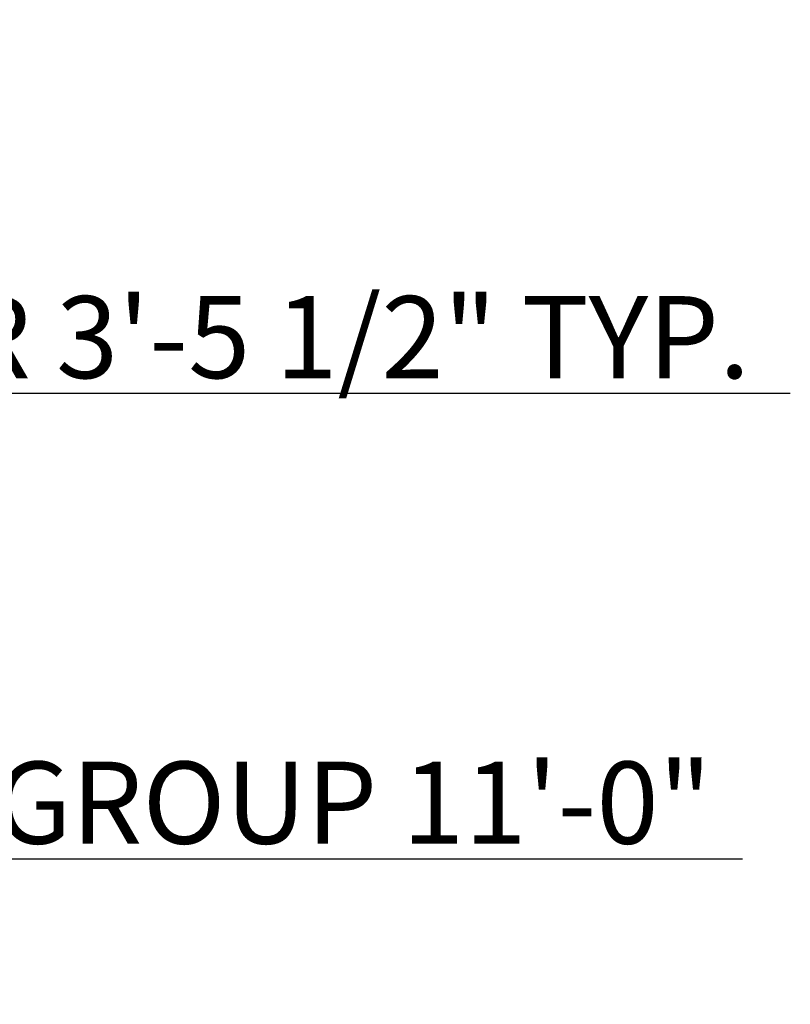
# Model space of a CAD drawing. Units: inches. Extents: x 597 to 1323, y 1833 to 2686.
# Tile 4 of 10: x 1158 to 1322, y 1957 to 2167. Entities that reach past the tile are written whole.
import ezdxf

# ---------------------------------------------------------------- set-up
doc = ezdxf.new("R2010")
doc.units = ezdxf.units.IN
doc.layers.add('A-ANNO-DIMS', color=2, linetype='Continuous', lineweight=18)
doc.styles.get("Standard").update_dxf_attribs({"font": 'arial.ttf'})
doc.dimstyles.new('ISO-25', dxfattribs={"dimtxt": 17.5, "dimasz": 2.5, "dimexe": 0, "dimexo": 0, "dimtad": 1, "dimdec": 1, "dimlunit": 3, "dimtxsty": 'Standard', "dimblk": 'OPEN90', "dimcen": 2.5, "dimadec": 0, "dimazin": 0, "dimtfac": 1, "dimtdec": 1, "dimtmove": 0, "dimatfit": 3, "dimfxl": 0, "dimfxlon": 1, "dimarcsym": 0})

# ---------------------------------------------------------------- blocks, each defined once
blk = doc.blocks.new('_Open90')
at = {"color": 0, "linetype": 'ByBlock', "lineweight": -2}
for p, q in [((0, 0), (-1, 0)), ((-0.5, 0.5), (0, 0)), ((0, 0), (-0.5, -0.5))]:
    blk.add_line(p, q, dxfattribs=at)
blk = doc.blocks.new('*D43')
at = {"layer": 'A-ANNO-DIMS', "color": 0, "lineweight": -2, "transparency": 16777216}
for p, q in [((939.8, 2087.21), (976.17, 2087.21)), ((978.67, 2087.21), (1321.98, 2087.21))]:
    blk.add_line(p, q, dxfattribs=at)
at = {"layer": 'Defpoints', "color": 0, "transparency": 16777216}
for p in [(978.67, 2087.21), (937.3, 2081.01), (978.67, 2081.01)]:
    blk.add_point(p, dxfattribs=at)
at = {"layer": 'A-ANNO-DIMS', "color": 0, "lineweight": -2, "transparency": 16777216, "xscale": 2.5, "yscale": 2.5, "zscale": 2.5, "rotation": 180}
blk.add_blockref('_Open90', (937.3, 2087.21), dxfattribs=at)
at = {"layer": 'A-ANNO-DIMS', "color": 0, "lineweight": -2, "transparency": 16777216, "xscale": 2.5, "yscale": 2.5, "zscale": 2.5}
blk.add_blockref('_Open90', (978.67, 2087.21), dxfattribs=at)
at = {"layer": 'A-ANNO-DIMS', "color": 0, "transparency": 16777216, "insert": (1151.58, 2096.9), "char_height": 17.5, "attachment_point": 5}
blk.add_mtext('LOUNGE CHAIR 3\'-5 1/2" TYP.', dxfattribs=at)
blk = doc.blocks.new('*D51')
at = {"layer": 'A-ANNO-DIMS', "color": 0, "lineweight": -2, "transparency": 16777216}
for p, q in [((948.81, 1987.99), (1075.69, 1987.99)), ((1078.19, 1987.99), (1311.77, 1987.99))]:
    blk.add_line(p, q, dxfattribs=at)
at = {"layer": 'Defpoints', "color": 0, "transparency": 16777216}
for p in [(946.31, 2007.77), (1078.19, 2007.77), (1078.19, 1987.99)]:
    blk.add_point(p, dxfattribs=at)
at = {"layer": 'A-ANNO-DIMS', "color": 0, "lineweight": -2, "transparency": 16777216, "xscale": 2.5, "yscale": 2.5, "zscale": 2.5, "rotation": 180}
blk.add_blockref('_Open90', (946.31, 1987.99), dxfattribs=at)
at = {"layer": 'A-ANNO-DIMS', "color": 0, "lineweight": -2, "transparency": 16777216, "xscale": 2.5, "yscale": 2.5, "zscale": 2.5}
blk.add_blockref('_Open90', (1078.19, 1987.99), dxfattribs=at)
at = {"layer": 'A-ANNO-DIMS', "color": 0, "transparency": 16777216, "insert": (1196.23, 1997.67), "char_height": 17.5, "attachment_point": 5}
blk.add_mtext('SOFA GROUP 11\'-0"', dxfattribs=at)

msp = doc.modelspace()

# ---------------------------------------------------------------- dimensions: what is measured, and where the dimension line sits
at = {"layer": 'A-ANNO-DIMS'}
for base, p1, p2, text, picture, middle in [((978.67, 2087.21), (937.3, 2081.01), (978.67, 2081.01), 'LOUNGE CHAIR <> TYP.', '*D43', (1151.58, 2096.9)), ((1078.19, 1987.99), (946.31, 2007.77), (1078.19, 2007.77), 'SOFA GROUP <>', '*D51', (1196.23, 1997.67))]:
    dim = msp.add_linear_dim(base=base, p1=p1, p2=p2, text=text, dimstyle='ISO-25', override={"dimdec": 1, "dimlfac": 1, "dimrnd": 0, "dimzin": 1, "dimdsep": 46, "dimlunit": 4, "dimfrac": 2}, dxfattribs=at)
    dim.commit()
    dim.dimension.update_dxf_attribs({"geometry": picture, "text_midpoint": middle})

doc.saveas('drawing.dxf')
